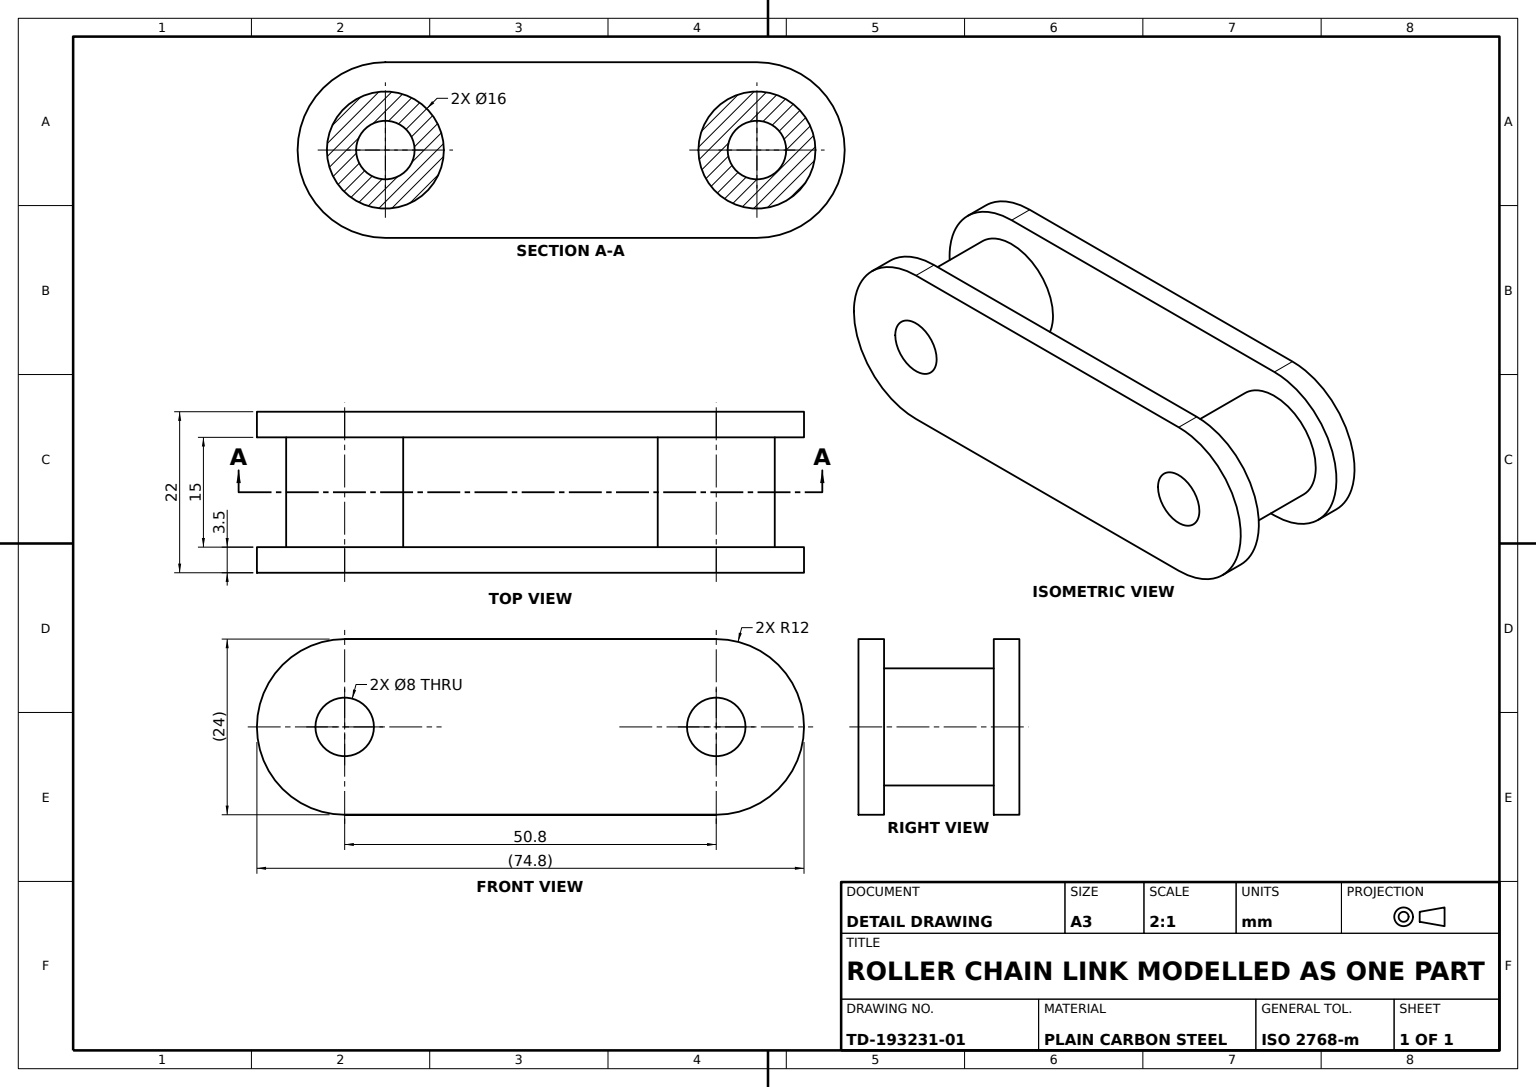
from build123d import *

# Parameters (mm, degrees)
REAR_LINK_PLATE_DEPTH  = 3.5
ROLLER_PROFILES_R      = 8
ROLLERS_2X_16_DEPTH    = 15
FRONT_LINK_PLATE_DEPTH = 3.5
PIN_BORE_PROFILES_R    = 4
PIN_BORES_2X_8_DEPTH   = 22


with BuildPart() as part:
    # Rear Plate Profile → Rear Link Plate (new body)
    with BuildSketch(Plane.XY):
        with BuildLine():
            Line((0, 12), (50.8, 12))
            ThreePointArc((50.8, 12), (62.8, 0), (50.8, -12))
            Line((50.8, -12), (0, -12))
            ThreePointArc((0, -12), (-12, 0), (0, 12))
        make_face()
    extrude(amount=REAR_LINK_PLATE_DEPTH)

    # Roller Profiles → Rollers 2xØ16 (add)
    with BuildSketch(Plane.XY.offset(3.5)):
        Circle(ROLLER_PROFILES_R)
        with Locations((50.8, 0)):
            Circle(ROLLER_PROFILES_R)
    extrude(amount=ROLLERS_2X_16_DEPTH)

    # Front Plate Profile → Front Link Plate (add)
    with BuildSketch(Plane.XY.offset(18.5)):
        with BuildLine():
            Line((0, 12), (50.8, 12))
            ThreePointArc((50.8, 12), (62.8, 0), (50.8, -12))
            Line((50.8, -12), (0, -12))
            ThreePointArc((0, -12), (-12, 0), (0, 12))
        make_face()
    extrude(amount=FRONT_LINK_PLATE_DEPTH)

    # Pin Bore Profiles → Pin Bores 2xØ8 (cut)
    with BuildSketch(Plane.XY.offset(22)):
        Circle(PIN_BORE_PROFILES_R)
        with Locations((50.8, 0)):
            Circle(PIN_BORE_PROFILES_R)
    extrude(amount=-PIN_BORES_2X_8_DEPTH, mode=Mode.SUBTRACT)


solid = part.part
